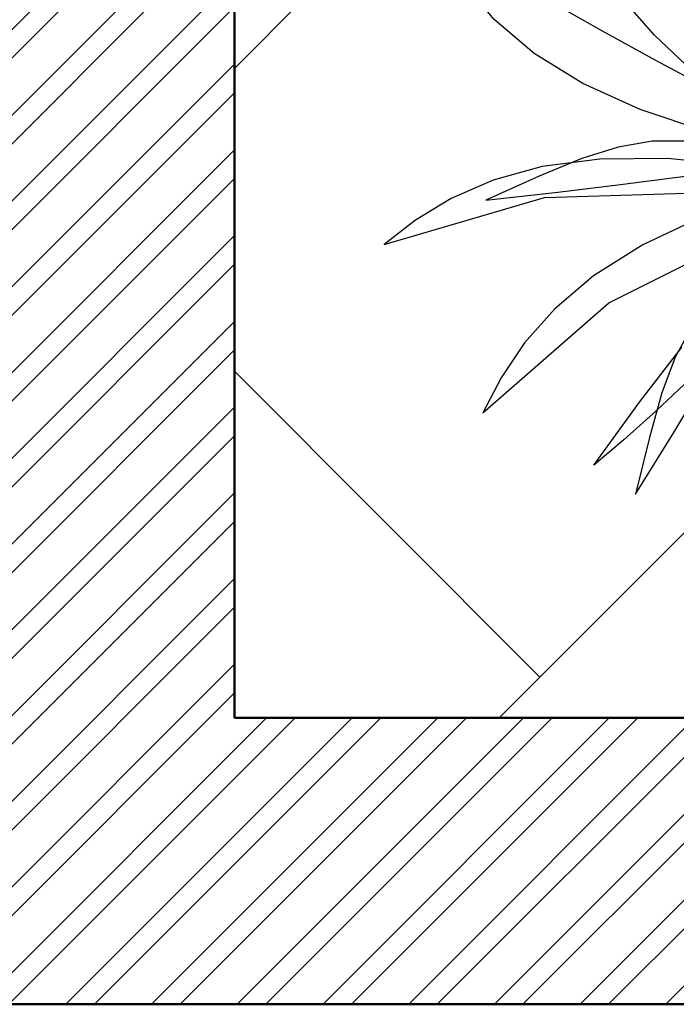
# Model space of a CAD drawing. Units: inches. Extents: x 3590 to 5167, y 65 to 1917.
# Tile 29 of 100: x 4927 to 4947, y 1326 to 1357. Entities that reach past the tile are written whole.
import ezdxf

# ---------------------------------------------------------------- set-up
doc = ezdxf.new("R2010")
doc.units = ezdxf.units.IN
for name, color, linetype, lineweight in [('A-FLOR-PATT', 8, 'Continuous', 13), ('A-WALL', 7, 'Continuous', 50), ('A-WALL-PATT', 251, 'Continuous', 13), ('L-PLNT', 94, 'Continuous', 18)]:
    doc.layers.add(name, color=color, linetype=linetype, lineweight=lineweight)
doc.layers.add('DIENHOA', color=3, linetype='Continuous')

# ---------------------------------------------------------------- blocks, each defined once
blk = doc.blocks.new('Cay03_mb')
at = {"layer": 'DIENHOA'}
for p, q in [((-254.7, 27.4), (-298.6, 20.1)), ((-208, 27.8), (-254.7, 27.4)), ((-298.6, 20.1), (-345, 5.4)), ((-345, 5.4), (-399.6, -17.1)), ((-225.8, -18.9), (-165.8, -11.3)), ((-399.6, -17.1), (-468, -47.9)), ((-295.3, -27.9), (-225.8, -18.9)), ((-468, -47.9), (-375.6, -37.8)), ((-375.6, -37.8), (-295.3, -27.9)), ((-271, -306.6), (-216.3, -235.6)), ((-206.3, -276.5), (-249.6, -317.8)), ((-329.5, -387.1), (-271, -306.6)), ((-249.6, -317.8), (-291, -354.7)), ((-291, -354.7), (-329.5, -387.1))]:
    blk.add_line(p, q, dxfattribs=at)
for points in [[(-16.4, -26.7), (-108.3, 38.6), (-186.9, 101.7), (-252.4, 163.5), (-305.1, 224.4), (-345.4, 285.2), (-373.7, 346.6), (-390.4, 409.2), (-395.6, 473.7)], [(-530.5, 289.7), (-458.3, 248.1), (-387.9, 207.8), (-318.9, 168.7), (-250.8, 131.1), (-182.9, 94.8), (-114.9, 59.9), (-46.2, 26.5), (23.7, -5.4)], [(23.7, -5.4), (-87.2, 15.2), (-185, 39.6), (-270.3, 68.2), (-343.7, 101.4), (-405.9, 139.7), (-457.3, 183.5), (-498.7, 233.4), (-530.5, 289.7)], [(-16.4, -26.7), (-134, -4.7), (-235.3, 5.3), (-322, 4.7), (-395.9, -5), (-458.7, -22.3), (-512.3, -45.7), (-558.2, -73.6), (-598.4, -104.7)], [(-471.9, -320.3), (-310.5, -179.3), (-97.7, -73.3), (23.7, -5.4)], [(23.7, -5.4), (-92.3, -34.8), (-188.4, -68.2), (-266.9, -105.1), (-329.9, -144.9), (-379.7, -187), (-418.5, -230.7), (-448.5, -275.3), (-471.9, -320.3)], [(-598.4, -104.7), (-392.7, -44.4), (-155, -37.4), (-16.4, -26.7)], [(-276.2, -424.4), (-227.3, -345.4), (-185.7, -276.1), (-150, -215.7), (-119.1, -163.8), (-91.5, -119.5), (-66, -82.3), (-41.4, -51.6), (-16.4, -26.7)], [(-16.4, -26.7), (-84.9, -86), (-137, -133.1), (-175.8, -173), (-204.3, -210), (-225.5, -249.1), (-242.5, -294.7), (-258.4, -351.6), (-276.2, -424.4)]]:
    blk.add_lwpolyline(points, dxfattribs=at)

msp = doc.modelspace()

# ---------------------------------------------------------------- hatches: boundary and pattern name
at = {"layer": 'A-FLOR-PATT', "transparency": 33554687}
h = msp.add_hatch(dxfattribs=at)
h.set_pattern_fill('AR-HBONE', color=256, scale=0.2)
h.set_pattern_definition([(45, (-588.972, 0), (0, 28.73682), [60.96, -20.32]), (135, (-574.604, 14.368), (3e-15, 28.73682), [60.96, -20.32])])
h.paths.add_polyline_path([(5071.274, 1796.999), (4933.274, 1796.999), (4933.274, 1753.999), (4962.774, 1753.999, -0.414214), (4928.774, 1719.999), (4933.274, 1718.999), (4933.274, 1334.999), (5071.274, 1334.999)])
h.paths.add_polyline_path([(4951.78, 1521.077), (4951.715, 1521.04), (4951.563, 1520.895)], flags=16)
h.paths.add_polyline_path([(4952.267, 1521.376), (4952.198, 1521.371), (4952.198, 1521.356)], flags=0)
h.paths.add_polyline_path([(4967.051, 1529.728), (4965.231, 1528.694), (4963.411, 1527.714), (4961.756, 1526.851), (4963.589, 1527.449), (4964.036, 1527.478), (4962.975, 1527.249), (4961.76, 1526.852), (4959.792, 1525.834), (4958.005, 1524.895), (4956.24, 1523.93), (4954.504, 1522.919), (4954.129, 1522.682), (4953.361, 1521.997), (4953.366, 1521.998), (4953.605, 1522.064), (4955.106, 1522.761), (4956.921, 1523.434), (4958.678, 1523.915), (4960.358, 1524.2), (4961.945, 1524.286), (4964.171, 1524.108), (4965.958, 1523.309), (4963.863, 1522.976), (4965.187, 1522.499), (4963.366, 1522.497), (4961.545, 1522.487), (4959.764, 1522.461), (4958.304, 1522.419), (4957.974, 1522.388), (4956.307, 1522.232), (4954.718, 1522.071), (4953.251, 1521.899), (4953.525, 1521.623), (4954.331, 1521.379), (4956.243, 1521.23), (4958.039, 1520.93), (4959.684, 1520.483), (4961.16, 1519.896), (4963.107, 1518.8), (4964.393, 1517.325), (4962.973, 1517.726), (4964.558, 1516.661), (4965.407, 1515.708), (4963.507, 1516.322), (4961.68, 1517.005), (4959.935, 1517.745), (4958.282, 1518.528), (4956.732, 1519.343), (4955.295, 1520.175), (4954.672, 1520.572), (4954.513, 1520.627), (4955.658, 1519.318), (4956.703, 1517.982), (4957.644, 1516.647), (4958.485, 1515.334), (4959.55, 1513.524), (4960.438, 1511.769), (4958.841, 1513.62), (4957.452, 1515.325), (4955.819, 1517.459), (4956.665, 1515.448), (4957.111, 1513.923), (4957.447, 1511.714), (4957.076, 1509.793), (4956.538, 1511.11), (4955.992, 1512.569), (4955.444, 1514.125), (4954.898, 1515.735), (4954.357, 1517.356), (4953.824, 1518.943), (4953.305, 1520.452), (4953.065, 1521.116), (4952.971, 1521.146), (4952.949, 1521.086), (4952.73, 1520.199), (4953.37, 1518.024), (4953.757, 1516.373), (4954.051, 1514.765), (4954.264, 1513.221), (4954.471, 1511.131), (4954.497, 1510.402), (4954.409, 1511.76), (4954.264, 1513.221), (4954.051, 1514.765), (4953.757, 1516.373), (4953.37, 1518.024), (4952.877, 1519.698), (4952.716, 1520.141), (4952.533, 1519.059), (4952.374, 1517.789), (4952.219, 1516.312), (4952.046, 1514.6), (4951.833, 1512.626), (4951.557, 1510.363), (4951.203, 1512.168), (4950.852, 1514.339), (4950.985, 1516.376), (4951.66, 1518.286), (4952.593, 1520.481), (4952.357, 1521.13), (4951.855, 1520.328), (4950.839, 1518.908), (4949.777, 1517.587), (4948.916, 1516.617), (4948.111, 1515.256), (4947.089, 1513.554), (4945.889, 1511.615), (4946.326, 1513.402), (4946.562, 1514.249), (4945.528, 1513.327), (4944.581, 1512.531), (4946.018, 1514.508), (4947.204, 1516.048), (4947.893, 1517.313), (4949.307, 1518.764), (4950.414, 1519.767), (4950.451, 1519.806), (4952.267, 1521.376), (4951.645, 1521.493), (4950.404, 1521.18), (4948.044, 1520.359), (4946.119, 1519.452), (4944.572, 1518.475), (4943.35, 1517.443), (4941.997, 1515.92), (4941.661, 1515.275), (4942.813, 1516.99), (4944.572, 1518.475), (4946.119, 1519.452), (4948.044, 1520.359), (4950.404, 1521.18), (4951.645, 1521.493), (4949.647, 1521.868), (4948.6, 1521.756), (4947.126, 1521.57), (4945.42, 1521.348), (4943.45, 1521.105), (4941.183, 1520.856), (4942.86, 1521.613), (4943.873, 1522.03), (4942.952, 1521.909), (4941.41, 1521.485), (4939.543, 1520.67), (4938.968, 1520.226), (4940.733, 1521.299), (4942.952, 1521.909), (4943.702, 1522.008), (4945.894, 1522.7), (4947.565, 1522.714), (4948.921, 1522.566), (4951.131, 1522.183), (4950.971, 1522.297), (4948.129, 1523.006), (4946.035, 1523.707), (4944.232, 1524.521), (4942.707, 1525.461), (4941.444, 1526.537), (4940.43, 1527.761), (4939.649, 1529.143), (4941.421, 1528.122), (4943.147, 1527.132), (4944.841, 1526.175), (4946.514, 1525.25), (4948.179, 1524.359), (4948.365, 1524.263), (4946.475, 1526.045), (4945.181, 1527.54), (4944.19, 1529.033), (4943.496, 1530.54), (4943.278, 1531.36), (4942.498, 1531.919), (4943.114, 1531.762), (4942.959, 1533.659), (4944.14, 1531.989), (4944.612, 1531.323), (4946.202, 1530.463), (4947.486, 1529.509), (4948.79, 1528.226), (4950.368, 1526.237), (4949.485, 1528.155), (4948.851, 1530.123), (4948.491, 1532.041), (4948.381, 1533.918), (4948.501, 1535.76), (4948.827, 1537.573), (4949.418, 1535.565), (4949.957, 1533.569), (4950.464, 1531.586), (4950.961, 1529.617), (4951.391, 1527.954), (4951.724, 1530.687), (4952.201, 1532.58), (4952.889, 1534.33), (4953.77, 1535.951), (4954.827, 1537.46), (4954.521, 1535.39), (4954.273, 1533.937), (4955.58, 1535.663), (4956.748, 1536.739), (4956.159, 1534.78), (4955.589, 1532.873), (4955.043, 1531.006), (4954.525, 1529.166), (4954.038, 1527.341), (4953.638, 1525.733), (4953.611, 1525.586), (4953.398, 1524.166), (4953.382, 1524.009), (4954.07, 1525.476), (4954.912, 1527.022), (4956.136, 1528.894), (4957.847, 1530.577), (4959.376, 1531.54), (4958.256, 1530.104), (4957.143, 1528.663), (4956.066, 1527.243), (4955.056, 1525.871), (4954.141, 1524.571), (4953.352, 1523.372), (4953.311, 1523.303), (4953.273, 1522.925), (4953.261, 1522.382), (4954.103, 1523.373), (4954.63, 1524.284), (4955.961, 1526.358), (4957.23, 1528.13), (4958.421, 1529.609), (4960.037, 1531.368), (4961.374, 1532.375), (4962.101, 1532.77), (4961.07, 1531.061), (4959.987, 1529.438), (4958.869, 1527.908), (4958.15, 1527.007), (4959.803, 1528.003), (4961.589, 1528.793), (4963.391, 1529.328), (4965.211, 1529.632)], flags=16)
h.paths.add_polyline_path([(4962.944, 1523.182), (4961.107, 1523.422), (4960.392, 1523.362), (4962.35, 1523.331)], flags=0)
h.paths.add_polyline_path([(5049.541, 1584.551), (5049.476, 1584.515), (5049.325, 1584.37)], flags=16)
h.paths.add_polyline_path([(5050.028, 1584.851), (5049.959, 1584.845), (5049.959, 1584.83)], flags=0)
h.paths.add_polyline_path([(5042.333, 1581.949), (5043.88, 1582.926), (5045.806, 1583.833), (5048.165, 1584.654), (5049.406, 1584.967), (5047.408, 1585.342), (5046.361, 1585.231), (5044.888, 1585.044), (5043.181, 1584.822), (5041.211, 1584.579), (5038.944, 1584.33), (5040.622, 1585.087), (5041.634, 1585.504), (5040.713, 1585.383), (5039.171, 1584.959), (5037.304, 1584.144), (5036.729, 1583.7), (5038.494, 1584.773), (5040.713, 1585.383), (5041.463, 1585.482), (5043.655, 1586.174), (5045.326, 1586.188), (5046.682, 1586.04), (5048.893, 1585.657), (5048.732, 1585.771), (5045.891, 1586.48), (5043.796, 1587.181), (5041.994, 1587.996), (5040.468, 1588.935), (5039.205, 1590.011), (5038.191, 1591.235), (5037.41, 1592.617), (5039.182, 1591.596), (5040.909, 1590.607), (5042.602, 1589.649), (5044.275, 1588.724), (5045.94, 1587.833), (5046.126, 1587.738), (5044.237, 1589.519), (5042.942, 1591.015), (5041.952, 1592.508), (5041.257, 1594.014), (5041.039, 1594.834), (5040.26, 1595.393), (5040.875, 1595.237), (5040.721, 1597.133), (5041.901, 1595.463), (5042.373, 1594.798), (5043.963, 1593.938), (5045.247, 1592.983), (5046.552, 1591.701), (5048.129, 1589.712), (5047.247, 1591.63), (5046.613, 1593.597), (5046.252, 1595.515), (5046.142, 1597.392), (5046.262, 1599.234), (5046.588, 1601.047), (5047.179, 1599.039), (5047.718, 1597.043), (5048.225, 1595.06), (5048.722, 1593.091), (5049.152, 1591.429), (5049.485, 1594.161), (5049.962, 1596.054), (5050.65, 1597.804), (5051.532, 1599.425), (5052.589, 1600.934), (5052.283, 1598.864), (5052.034, 1597.411), (5053.341, 1599.137), (5054.509, 1600.213), (5053.92, 1598.254), (5053.35, 1596.348), (5052.805, 1594.48), (5052.286, 1592.64), (5051.799, 1590.815), (5051.4, 1589.207), (5051.373, 1589.06), (5051.159, 1587.64), (5051.143, 1587.483), (5051.831, 1588.95), (5052.673, 1590.496), (5053.898, 1592.368), (5055.608, 1594.051), (5057.137, 1595.014), (5056.017, 1593.578), (5054.904, 1592.137), (5053.828, 1590.717), (5052.817, 1589.345), (5051.902, 1588.046), (5051.113, 1586.846), (5051.072, 1586.777), (5051.034, 1586.399), (5051.022, 1585.856), (5051.864, 1586.847), (5052.391, 1587.758), (5053.723, 1589.832), (5054.991, 1591.604), (5056.182, 1593.083), (5057.798, 1594.842), (5059.135, 1595.849), (5059.863, 1596.244), (5058.831, 1594.535), (5057.749, 1592.912), (5056.63, 1591.382), (5055.912, 1590.482), (5057.564, 1591.477), (5059.35, 1592.267), (5061.152, 1592.802), (5062.972, 1593.106), (5064.812, 1593.203), (5062.992, 1592.169), (5061.172, 1591.188), (5059.518, 1590.325), (5061.35, 1590.924), (5061.797, 1590.952), (5060.737, 1590.723), (5059.521, 1590.326), (5057.553, 1589.308), (5055.766, 1588.369), (5054.002, 1587.404), (5052.265, 1586.393), (5051.891, 1586.156), (5051.122, 1585.471), (5051.127, 1585.472), (5051.366, 1585.538), (5052.867, 1586.235), (5054.682, 1586.908), (5056.439, 1587.389), (5058.12, 1587.675), (5059.706, 1587.76), (5061.933, 1587.583), (5063.719, 1586.783), (5061.624, 1586.45), (5062.949, 1585.973), (5061.127, 1585.971), (5059.307, 1585.961), (5057.525, 1585.935), (5056.065, 1585.893), (5055.735, 1585.862), (5054.068, 1585.707), (5052.479, 1585.546), (5051.012, 1585.373), (5051.286, 1585.097), (5052.092, 1584.853), (5054.004, 1584.704), (5055.8, 1584.404), (5057.446, 1583.958), (5058.921, 1583.37), (5060.868, 1582.274), (5062.154, 1580.799), (5060.734, 1581.2), (5062.32, 1580.135), (5063.168, 1579.182), (5061.269, 1579.796), (5059.441, 1580.479), (5057.696, 1581.219), (5056.043, 1582.003), (5054.493, 1582.817), (5053.057, 1583.649), (5052.433, 1584.047), (5052.274, 1584.101), (5053.42, 1582.793), (5054.464, 1581.457), (5055.405, 1580.121), (5056.247, 1578.809), (5057.311, 1576.998), (5058.199, 1575.244), (5056.602, 1577.094), (5055.213, 1578.799), (5053.58, 1580.933), (5054.427, 1578.922), (5054.872, 1577.397), (5055.208, 1575.189), (5054.838, 1573.267), (5054.299, 1574.584), (5053.754, 1576.043), (5053.206, 1577.599), (5052.659, 1579.209), (5052.118, 1580.83), (5051.585, 1582.417), (5051.066, 1583.927), (5050.826, 1584.59), (5050.733, 1584.62), (5050.711, 1584.561), (5050.491, 1583.673), (5051.131, 1581.498), (5051.518, 1579.847), (5051.813, 1578.24), (5052.026, 1576.695), (5052.233, 1574.605), (5052.258, 1573.876), (5052.17, 1575.234), (5052.026, 1576.695), (5051.813, 1578.24), (5051.518, 1579.847), (5051.131, 1581.498), (5050.638, 1583.172), (5050.477, 1583.615), (5050.294, 1582.533), (5050.136, 1581.263), (5049.981, 1579.786), (5049.807, 1578.074), (5049.594, 1576.1), (5049.318, 1573.837), (5048.965, 1575.642), (5048.613, 1577.813), (5048.747, 1579.85), (5049.421, 1581.76), (5050.354, 1583.955), (5050.118, 1584.604), (5049.616, 1583.802), (5048.6, 1582.382), (5047.538, 1581.061), (5046.677, 1580.091), (5045.872, 1578.73), (5044.85, 1577.028), (5043.651, 1575.089), (5044.087, 1576.877), (5044.324, 1577.723), (5043.289, 1576.801), (5042.342, 1576.005), (5043.779, 1577.982), (5044.966, 1579.522), (5045.655, 1580.787), (5047.068, 1582.239), (5048.175, 1583.241), (5048.213, 1583.28), (5050.028, 1584.851), (5049.406, 1584.967), (5048.165, 1584.654), (5045.806, 1583.833), (5043.88, 1582.926), (5042.333, 1581.949), (5041.111, 1580.917), (5039.758, 1579.394), (5039.423, 1578.749), (5040.575, 1580.464)], flags=16)
h.paths.add_polyline_path([(4954.799, 1533.12), (4954.262, 1532.079), (4953.831, 1530.935), (4953.505, 1529.636), (4953.283, 1528.133), (4953.167, 1526.376), (4953.156, 1524.315), (4953.277, 1521.236), (4952.802, 1521.842), (4951.557, 1521.998), (4950.976, 1521.961), (4952.661, 1521.941), (4952.802, 1521.842), (4953.152, 1523.593), (4953.167, 1526.376), (4953.283, 1528.133), (4953.609, 1530.346), (4954.456, 1532.592)], flags=0)
h.paths.add_polyline_path([(5050.563, 1585.316), (5049.318, 1585.472), (5048.737, 1585.435), (5050.422, 1585.415), (5050.563, 1585.316), (5050.914, 1587.067), (5050.928, 1589.851), (5051.045, 1591.607), (5051.371, 1593.82), (5052.217, 1596.066), (5052.56, 1596.594), (5052.024, 1595.554), (5051.592, 1594.409), (5051.266, 1593.11), (5051.045, 1591.607), (5050.928, 1589.851), (5050.918, 1587.789), (5051.038, 1584.71)], flags=0)
h.paths.add_polyline_path([(5058.153, 1586.836), (5060.111, 1586.805), (5060.705, 1586.656), (5058.868, 1586.896)], flags=0)
h.paths.add_polyline_path([(5049.541, 1430.936), (5049.476, 1430.9), (5049.325, 1430.755)], flags=16)
h.paths.add_polyline_path([(5050.028, 1431.236), (5049.959, 1431.231), (5049.959, 1431.215)], flags=0)
h.paths.add_polyline_path([(5046.588, 1447.432), (5047.179, 1445.425), (5047.718, 1443.429), (5048.225, 1441.446), (5048.722, 1439.476), (5049.152, 1437.814), (5049.485, 1440.546), (5049.962, 1442.439), (5050.65, 1444.189), (5051.532, 1445.811), (5052.589, 1447.319), (5052.283, 1445.249), (5052.034, 1443.796), (5053.341, 1445.522), (5054.509, 1446.598), (5053.92, 1444.64), (5053.35, 1442.733), (5052.805, 1440.865), (5052.286, 1439.025), (5051.799, 1437.201), (5051.4, 1435.592), (5051.373, 1435.445), (5051.159, 1434.025), (5051.143, 1433.868), (5051.831, 1435.335), (5052.673, 1436.881), (5053.898, 1438.753), (5055.608, 1440.436), (5057.137, 1441.4), (5056.017, 1439.963), (5054.904, 1438.522), (5053.828, 1437.102), (5052.817, 1435.73), (5051.902, 1434.431), (5051.113, 1433.231), (5051.072, 1433.162), (5051.034, 1432.784), (5051.022, 1432.242), (5051.864, 1433.232), (5052.391, 1434.143), (5053.723, 1436.217), (5054.991, 1437.989), (5056.182, 1439.468), (5057.798, 1441.227), (5059.135, 1442.235), (5059.863, 1442.629), (5058.831, 1440.921), (5057.749, 1439.298), (5056.63, 1437.767), (5055.912, 1436.867), (5057.564, 1437.863), (5059.35, 1438.652), (5061.152, 1439.187), (5062.972, 1439.491), (5064.812, 1439.588), (5062.992, 1438.554), (5061.172, 1437.573), (5059.518, 1436.71), (5061.35, 1437.309), (5061.797, 1437.337), (5060.737, 1437.108), (5059.521, 1436.711), (5057.553, 1435.693), (5055.766, 1434.754), (5054.002, 1433.789), (5052.265, 1432.778), (5051.891, 1432.541), (5051.122, 1431.856), (5051.127, 1431.857), (5051.366, 1431.923), (5052.867, 1432.62), (5054.682, 1433.293), (5056.439, 1433.775), (5058.12, 1434.06), (5059.706, 1434.145), (5061.933, 1433.968), (5063.719, 1433.168), (5061.624, 1432.835), (5062.949, 1432.358), (5061.127, 1432.357), (5059.307, 1432.346), (5057.525, 1432.32), (5056.065, 1432.278), (5055.735, 1432.248), (5054.068, 1432.092), (5052.479, 1431.931), (5051.012, 1431.759), (5051.286, 1431.482), (5052.092, 1431.238), (5054.004, 1431.089), (5055.8, 1430.789), (5057.446, 1430.343), (5058.921, 1429.755), (5060.868, 1428.66), (5062.154, 1427.185), (5060.734, 1427.585), (5062.32, 1426.52), (5063.168, 1425.567), (5061.269, 1426.181), (5059.441, 1426.865), (5057.696, 1427.604), (5056.043, 1428.388), (5054.493, 1429.202), (5053.057, 1430.034), (5052.433, 1430.432), (5052.274, 1430.487), (5053.42, 1429.178), (5054.464, 1427.842), (5055.405, 1426.506), (5056.247, 1425.194), (5057.311, 1423.383), (5058.199, 1421.629), (5056.602, 1423.479), (5055.213, 1425.184), (5053.58, 1427.318), (5054.427, 1425.307), (5054.872, 1423.782), (5055.208, 1421.574), (5054.838, 1419.652), (5054.299, 1420.97), (5053.754, 1422.428), (5053.206, 1423.984), (5052.659, 1425.595), (5052.118, 1427.215), (5051.585, 1428.802), (5051.066, 1430.312), (5050.826, 1430.975), (5050.733, 1431.005), (5050.711, 1430.946), (5050.491, 1430.058), (5051.131, 1427.883), (5051.518, 1426.232), (5051.813, 1424.625), (5052.026, 1423.081), (5052.233, 1420.991), (5052.258, 1420.261), (5052.17, 1421.619), (5052.026, 1423.081), (5051.813, 1424.625), (5051.518, 1426.232), (5051.131, 1427.883), (5050.638, 1429.558), (5050.477, 1430.001), (5050.294, 1428.918), (5050.136, 1427.648), (5049.981, 1426.171), (5049.807, 1424.459), (5049.594, 1422.485), (5049.318, 1420.222), (5048.965, 1422.028), (5048.613, 1424.199), (5048.747, 1426.235), (5049.421, 1428.146), (5050.354, 1430.34), (5050.118, 1430.989), (5049.616, 1430.187), (5048.6, 1428.768), (5047.538, 1427.446), (5046.677, 1426.477), (5045.872, 1425.116), (5044.85, 1423.413), (5043.651, 1421.474), (5044.087, 1423.262), (5044.324, 1424.109), (5043.289, 1423.186), (5042.342, 1422.391), (5043.779, 1424.368), (5044.966, 1425.907), (5045.655, 1427.173), (5047.068, 1428.624), (5048.175, 1429.627), (5048.213, 1429.666), (5050.028, 1431.236), (5049.406, 1431.353), (5048.165, 1431.039), (5045.806, 1430.218), (5043.88, 1429.311), (5042.333, 1428.334), (5041.111, 1427.302), (5039.758, 1425.779), (5039.423, 1425.134), (5040.575, 1426.849), (5042.333, 1428.334), (5043.88, 1429.311), (5045.806, 1430.218), (5048.165, 1431.039), (5049.406, 1431.353), (5047.408, 1431.727), (5046.361, 1431.616), (5044.888, 1431.429), (5043.181, 1431.207), (5041.211, 1430.964), (5038.944, 1430.715), (5040.622, 1431.472), (5041.634, 1431.89), (5040.713, 1431.769), (5039.171, 1431.345), (5037.304, 1430.53), (5036.729, 1430.085), (5038.494, 1431.158), (5040.713, 1431.769), (5041.463, 1431.867), (5043.655, 1432.559), (5045.326, 1432.573), (5046.682, 1432.425), (5048.893, 1432.042), (5048.732, 1432.156), (5045.891, 1432.865), (5043.796, 1433.566), (5041.994, 1434.381), (5040.468, 1435.321), (5039.205, 1436.396), (5038.191, 1437.62), (5037.41, 1439.002), (5039.182, 1437.982), (5040.909, 1436.992), (5042.602, 1436.034), (5044.275, 1435.109), (5045.94, 1434.218), (5046.126, 1434.123), (5044.237, 1435.904), (5042.942, 1437.4), (5041.952, 1438.893), (5041.257, 1440.399), (5041.039, 1441.219), (5040.26, 1441.778), (5040.875, 1441.622), (5040.721, 1443.518), (5041.901, 1441.848), (5042.373, 1441.183), (5043.963, 1440.323), (5045.247, 1439.369), (5046.552, 1438.086), (5048.129, 1436.097), (5047.247, 1438.015), (5046.613, 1439.982), (5046.252, 1441.901), (5046.142, 1443.778), (5046.262, 1445.619)], flags=16)
h.paths.add_polyline_path([(5052.382, 1444.255), (5051.623, 1442.78), (5052.024, 1441.939), (5052.56, 1442.98)], flags=0)
h.paths.add_polyline_path([(5050.563, 1431.701), (5049.318, 1431.857), (5048.737, 1431.821), (5050.422, 1431.8)], flags=0)
h.paths.add_polyline_path([(5058.153, 1433.221), (5060.111, 1433.19), (5060.705, 1433.041), (5058.868, 1433.281)], flags=0)
h.paths.add_polyline_path([(5049.541, 1352.285), (5049.476, 1352.249), (5049.325, 1352.104)], flags=16)
h.paths.add_polyline_path([(5050.028, 1352.585), (5049.959, 1352.58), (5049.959, 1352.564)], flags=0)
h.paths.add_polyline_path([(5046.588, 1368.781), (5047.179, 1366.774), (5047.718, 1364.778), (5048.225, 1362.795), (5048.722, 1360.825), (5049.152, 1359.163), (5049.485, 1361.896), (5049.962, 1363.789), (5050.65, 1365.538), (5051.532, 1367.16), (5052.589, 1368.669), (5052.283, 1366.598), (5052.034, 1365.145), (5053.341, 1366.871), (5054.509, 1367.947), (5053.92, 1365.989), (5053.35, 1364.082), (5052.805, 1362.214), (5052.286, 1360.374), (5051.799, 1358.55), (5051.4, 1356.942), (5051.373, 1356.794), (5051.159, 1355.374), (5051.143, 1355.218), (5051.831, 1356.684), (5052.673, 1358.23), (5053.898, 1360.102), (5055.608, 1361.786), (5057.137, 1362.749), (5056.017, 1361.313), (5054.904, 1359.872), (5053.828, 1358.452), (5052.817, 1357.079), (5051.902, 1355.78), (5051.113, 1354.581), (5051.072, 1354.512), (5051.034, 1354.133), (5051.022, 1353.591), (5051.864, 1354.581), (5052.391, 1355.492), (5053.723, 1357.566), (5054.991, 1359.338), (5056.182, 1360.817), (5057.798, 1362.577), (5059.135, 1363.584), (5059.863, 1363.979), (5058.831, 1362.27), (5057.749, 1360.647), (5056.63, 1359.117), (5055.912, 1358.216), (5057.564, 1359.212), (5059.35, 1360.001), (5061.152, 1360.536), (5062.972, 1360.841), (5064.812, 1360.937), (5062.992, 1359.903), (5061.172, 1358.923), (5059.518, 1358.059), (5061.35, 1358.658), (5061.797, 1358.687), (5060.737, 1358.458), (5059.521, 1358.061), (5057.553, 1357.043), (5055.766, 1356.103), (5054.002, 1355.138), (5052.265, 1354.127), (5051.891, 1353.89), (5051.122, 1353.206), (5051.127, 1353.206), (5051.366, 1353.272), (5052.867, 1353.969), (5054.682, 1354.643), (5056.439, 1355.124), (5058.12, 1355.409), (5059.706, 1355.495), (5061.933, 1355.317), (5063.719, 1354.518), (5061.624, 1354.184), (5062.949, 1353.708), (5061.127, 1353.706), (5059.307, 1353.695), (5057.525, 1353.669), (5056.065, 1353.627), (5055.735, 1353.597), (5054.068, 1353.441), (5052.479, 1353.28), (5051.012, 1353.108), (5051.286, 1352.831), (5052.092, 1352.587), (5054.004, 1352.439), (5055.8, 1352.138), (5057.446, 1351.692), (5058.921, 1351.104), (5060.868, 1350.009), (5062.154, 1348.534), (5060.734, 1348.935), (5062.32, 1347.869), (5063.168, 1346.916), (5061.269, 1347.53), (5059.441, 1348.214), (5057.696, 1348.954), (5056.043, 1349.737), (5054.493, 1350.551), (5053.057, 1351.383), (5052.433, 1351.781), (5052.274, 1351.836), (5053.42, 1350.527), (5054.464, 1349.191), (5055.405, 1347.855), (5056.247, 1346.543), (5057.311, 1344.733), (5058.199, 1342.978), (5056.602, 1344.828), (5055.213, 1346.534), (5053.58, 1348.667), (5054.427, 1346.656), (5054.872, 1345.132), (5055.208, 1342.923), (5054.838, 1341.002), (5054.299, 1342.319), (5053.754, 1343.778), (5053.206, 1345.334), (5052.659, 1346.944), (5052.118, 1348.564), (5051.585, 1350.151), (5051.066, 1351.661), (5050.826, 1352.324), (5050.733, 1352.355), (5050.711, 1352.295), (5050.491, 1351.408), (5051.131, 1349.232), (5051.518, 1347.581), (5051.813, 1345.974), (5052.026, 1344.43), (5052.233, 1342.34), (5052.258, 1341.61), (5052.17, 1342.969), (5052.026, 1344.43), (5051.813, 1345.974), (5051.518, 1347.581), (5051.131, 1349.232), (5050.638, 1350.907), (5050.477, 1351.35), (5050.294, 1350.267), (5050.136, 1348.997), (5049.981, 1347.52), (5049.807, 1345.809), (5049.594, 1343.835), (5049.318, 1341.571), (5048.965, 1343.377), (5048.613, 1345.548), (5048.747, 1347.585), (5049.421, 1349.495), (5050.354, 1351.689), (5050.118, 1352.339), (5049.616, 1351.536), (5048.6, 1350.117), (5047.538, 1348.795), (5046.677, 1347.826), (5045.872, 1346.465), (5044.85, 1344.763), (5043.651, 1342.824), (5044.087, 1344.611), (5044.324, 1345.458), (5043.289, 1344.535), (5042.342, 1343.74), (5043.779, 1345.717), (5044.966, 1347.256), (5045.655, 1348.522), (5047.068, 1349.973), (5048.175, 1350.976), (5048.213, 1351.015), (5050.028, 1352.585), (5049.406, 1352.702), (5048.165, 1352.388), (5045.806, 1351.567), (5043.88, 1350.661), (5042.333, 1349.683), (5041.111, 1348.651), (5039.758, 1347.128), (5039.423, 1346.483), (5040.575, 1348.198), (5042.333, 1349.683), (5043.88, 1350.661), (5045.806, 1351.567), (5048.165, 1352.388), (5049.406, 1352.702), (5047.408, 1353.076), (5046.361, 1352.965), (5044.888, 1352.779), (5043.181, 1352.556), (5041.211, 1352.313), (5038.944, 1352.065), (5040.622, 1352.821), (5041.634, 1353.239), (5040.713, 1353.118), (5039.171, 1352.694), (5037.304, 1351.879), (5036.729, 1351.434), (5038.494, 1352.508), (5040.713, 1353.118), (5041.463, 1353.216), (5043.655, 1353.909), (5045.326, 1353.923), (5046.682, 1353.774), (5048.893, 1353.391), (5048.732, 1353.506), (5045.891, 1354.214), (5043.796, 1354.915), (5041.994, 1355.73), (5040.468, 1356.67), (5039.205, 1357.746), (5038.191, 1358.969), (5037.41, 1360.352), (5039.182, 1359.331), (5040.909, 1358.341), (5042.602, 1357.383), (5044.275, 1356.458), (5045.94, 1355.567), (5046.126, 1355.472), (5044.237, 1357.253), (5042.942, 1358.749), (5041.952, 1360.242), (5041.257, 1361.748), (5041.039, 1362.568), (5040.26, 1363.128), (5040.875, 1362.971), (5040.721, 1364.867), (5041.901, 1363.197), (5042.373, 1362.532), (5043.963, 1361.672), (5045.247, 1360.718), (5046.552, 1359.435), (5048.129, 1357.446), (5047.247, 1359.364), (5046.613, 1361.331), (5046.252, 1363.25), (5046.142, 1365.127), (5046.262, 1366.969)], flags=16)
h.paths.add_polyline_path([(5052.382, 1365.604), (5051.623, 1364.129), (5052.024, 1363.288), (5052.56, 1364.329)], flags=0)
h.paths.add_polyline_path([(4951.78, 1698.041), (4951.715, 1698.005), (4951.563, 1697.859)], flags=16)
h.paths.add_polyline_path([(4952.267, 1698.341), (4952.198, 1698.335), (4952.198, 1698.32)], flags=0)
h.paths.add_polyline_path([(4957.076, 1686.757), (4956.538, 1688.074), (4955.992, 1689.533), (4955.444, 1691.089), (4954.898, 1692.699), (4954.357, 1694.32), (4953.824, 1695.907), (4953.305, 1697.417), (4953.065, 1698.08), (4952.971, 1698.11), (4952.949, 1698.051), (4952.73, 1697.163), (4953.37, 1694.988), (4953.757, 1693.337), (4954.051, 1691.729), (4954.264, 1690.185), (4954.471, 1688.095), (4954.497, 1687.366), (4954.409, 1688.724), (4954.264, 1690.185), (4954.051, 1691.729), (4953.757, 1693.337), (4953.37, 1694.988), (4952.877, 1696.662), (4952.716, 1697.105), (4952.533, 1696.023), (4952.374, 1694.753), (4952.219, 1693.276), (4952.046, 1691.564), (4951.833, 1689.59), (4951.557, 1687.327), (4951.203, 1689.132), (4950.852, 1691.303), (4950.985, 1693.34), (4951.66, 1695.25), (4952.593, 1697.445), (4952.357, 1698.094), (4951.855, 1697.292), (4950.839, 1695.872), (4949.777, 1694.551), (4948.916, 1693.581), (4948.111, 1692.22), (4947.089, 1690.518), (4945.889, 1688.579), (4946.326, 1690.366), (4946.562, 1691.213), (4945.528, 1690.291), (4944.581, 1689.495), (4946.018, 1691.472), (4947.204, 1693.012), (4947.893, 1694.277), (4949.307, 1695.729), (4950.414, 1696.731), (4950.451, 1696.77), (4952.267, 1698.341), (4951.645, 1698.457), (4950.404, 1698.144), (4948.044, 1697.323), (4946.119, 1696.416), (4944.572, 1695.439), (4943.35, 1694.407), (4941.997, 1692.884), (4941.661, 1692.239), (4942.813, 1693.954), (4944.572, 1695.439), (4946.119, 1696.416), (4948.044, 1697.323), (4950.404, 1698.144), (4951.645, 1698.457), (4949.647, 1698.832), (4948.6, 1698.72), (4947.126, 1698.534), (4945.42, 1698.312), (4943.45, 1698.069), (4941.183, 1697.82), (4942.86, 1698.577), (4943.873, 1698.994), (4942.952, 1698.873), (4941.41, 1698.449), (4939.543, 1697.634), (4938.968, 1697.19), (4940.733, 1698.263), (4942.952, 1698.873), (4943.702, 1698.972), (4945.894, 1699.664), (4947.565, 1699.678), (4948.921, 1699.53), (4951.131, 1699.147), (4950.971, 1699.261), (4948.129, 1699.97), (4946.035, 1700.671), (4944.232, 1701.486), (4942.707, 1702.425), (4941.444, 1703.501), (4940.43, 1704.725), (4939.649, 1706.107), (4941.421, 1705.086), (4943.147, 1704.097), (4944.841, 1703.139), (4946.514, 1702.214), (4948.179, 1701.323), (4948.365, 1701.227), (4946.475, 1703.009), (4945.181, 1704.505), (4944.19, 1705.997), (4943.496, 1707.504), (4943.278, 1708.324), (4942.498, 1708.883), (4943.114, 1708.727), (4942.959, 1710.623), (4944.14, 1708.953), (4944.612, 1708.287), (4946.202, 1707.428), (4947.486, 1706.473), (4948.79, 1705.191), (4950.368, 1703.202), (4949.485, 1705.12), (4948.851, 1707.087), (4948.491, 1709.005), (4948.381, 1710.882), (4948.501, 1712.724), (4948.827, 1714.537), (4949.418, 1712.529), (4949.957, 1710.533), (4950.464, 1708.55), (4950.961, 1706.581), (4951.391, 1704.919), (4951.724, 1707.651), (4952.201, 1709.544), (4952.889, 1711.294), (4953.77, 1712.915), (4954.827, 1714.424), (4954.521, 1712.354), (4954.273, 1710.901), (4955.58, 1712.627), (4956.748, 1713.703), (4956.159, 1711.744), (4955.589, 1709.837), (4955.043, 1707.97), (4954.525, 1706.13), (4954.038, 1704.305), (4953.638, 1702.697), (4953.611, 1702.55), (4953.398, 1701.13), (4953.382, 1700.973), (4954.07, 1702.44), (4954.912, 1703.986), (4956.136, 1705.858), (4957.847, 1707.541), (4959.376, 1708.504), (4958.256, 1707.068), (4957.143, 1705.627), (4956.066, 1704.207), (4955.056, 1702.835), (4954.141, 1701.536), (4953.352, 1700.336), (4953.311, 1700.267), (4953.273, 1699.889), (4953.261, 1699.346), (4954.103, 1700.337), (4954.63, 1701.248), (4955.961, 1703.322), (4957.23, 1705.094), (4958.421, 1706.573), (4960.037, 1708.332), (4961.374, 1709.339), (4962.101, 1709.734), (4961.07, 1708.025), (4959.987, 1706.402), (4958.869, 1704.872), (4958.15, 1703.972), (4959.803, 1704.967), (4961.589, 1705.757), (4963.391, 1706.292), (4965.211, 1706.596), (4967.051, 1706.692), (4965.231, 1705.659), (4963.411, 1704.678), (4961.756, 1703.815), (4963.589, 1704.413), (4964.036, 1704.442), (4962.975, 1704.213), (4961.76, 1703.816), (4959.792, 1702.798), (4958.005, 1701.859), (4956.24, 1700.894), (4954.504, 1699.883), (4954.129, 1699.646), (4953.361, 1698.961), (4953.366, 1698.962), (4953.605, 1699.028), (4955.106, 1699.725), (4956.921, 1700.398), (4958.678, 1700.879), (4960.358, 1701.164), (4961.945, 1701.25), (4964.171, 1701.073), (4965.958, 1700.273), (4963.863, 1699.94), (4965.187, 1699.463), (4963.366, 1699.461), (4961.545, 1699.451), (4959.764, 1699.425), (4958.304, 1699.383), (4957.974, 1699.352), (4956.307, 1699.197), (4954.718, 1699.036), (4953.251, 1698.863), (4953.525, 1698.587), (4954.331, 1698.343), (4956.243, 1698.194), (4958.039, 1697.894), (4959.684, 1697.447), (4961.16, 1696.86), (4963.107, 1695.764), (4964.393, 1694.289), (4962.973, 1694.69), (4964.558, 1693.625), (4965.407, 1692.672), (4963.507, 1693.286), (4961.68, 1693.969), (4959.935, 1694.709), (4958.282, 1695.492), (4956.732, 1696.307), (4955.295, 1697.139), (4954.672, 1697.536), (4954.513, 1697.591), (4955.658, 1696.282), (4956.703, 1694.946), (4957.644, 1693.611), (4958.485, 1692.298), (4959.55, 1690.488), (4960.438, 1688.733), (4958.841, 1690.584), (4957.452, 1692.289), (4955.819, 1694.423), (4956.665, 1692.412), (4957.111, 1690.887), (4957.447, 1688.678)], flags=16)
h.paths.add_polyline_path([(5050.563, 1353.05), (5049.318, 1353.207), (5048.737, 1353.17), (5050.422, 1353.15)], flags=0)
h.paths.add_polyline_path([(4951.78, 1351.486), (4951.715, 1351.45), (4951.563, 1351.305)], flags=16)
h.paths.add_polyline_path([(4952.267, 1351.786), (4952.198, 1351.78), (4952.198, 1351.765)], flags=0)
h.paths.add_polyline_path([(4954.827, 1367.869), (4954.521, 1365.799), (4954.273, 1364.346), (4955.58, 1366.072), (4956.748, 1367.148), (4956.159, 1365.19), (4955.589, 1363.283), (4955.043, 1361.415), (4954.525, 1359.575), (4954.038, 1357.751), (4953.638, 1356.142), (4953.611, 1355.995), (4953.398, 1354.575), (4953.382, 1354.418), (4954.07, 1355.885), (4954.912, 1357.431), (4956.136, 1359.303), (4957.847, 1360.986), (4959.376, 1361.95), (4958.256, 1360.513), (4957.143, 1359.072), (4956.066, 1357.652), (4955.056, 1356.28), (4954.141, 1354.981), (4953.352, 1353.781), (4953.311, 1353.712), (4953.273, 1353.334), (4953.261, 1352.792), (4954.103, 1353.782), (4954.63, 1354.693), (4955.961, 1356.767), (4957.23, 1358.539), (4958.421, 1360.018), (4960.037, 1361.777), (4961.374, 1362.785), (4962.101, 1363.179), (4961.07, 1361.471), (4959.987, 1359.848), (4958.869, 1358.317), (4958.15, 1357.417), (4959.803, 1358.413), (4961.589, 1359.202), (4963.391, 1359.737), (4965.211, 1360.041), (4967.051, 1360.138), (4965.231, 1359.104), (4963.411, 1358.123), (4961.756, 1357.26), (4963.589, 1357.859), (4964.036, 1357.887), (4962.975, 1357.658), (4961.76, 1357.261), (4959.792, 1356.243), (4958.005, 1355.304), (4956.24, 1354.339), (4954.504, 1353.328), (4954.129, 1353.091), (4953.361, 1352.406), (4953.366, 1352.407), (4953.605, 1352.473), (4955.106, 1353.17), (4956.921, 1353.843), (4958.678, 1354.325), (4960.358, 1354.61), (4961.945, 1354.695), (4964.171, 1354.518), (4965.958, 1353.718), (4963.863, 1353.385), (4965.187, 1352.908), (4963.366, 1352.907), (4961.545, 1352.896), (4959.764, 1352.87), (4958.304, 1352.828), (4957.974, 1352.798), (4956.307, 1352.642), (4954.718, 1352.481), (4953.251, 1352.309), (4953.525, 1352.032), (4954.331, 1351.788), (4956.243, 1351.639), (4958.039, 1351.339), (4959.684, 1350.893), (4961.16, 1350.305), (4963.107, 1349.21), (4964.393, 1347.735), (4962.973, 1348.135), (4964.558, 1347.07), (4965.407, 1346.117), (4963.507, 1346.731), (4961.68, 1347.414), (4959.935, 1348.154), (4958.282, 1348.938), (4956.732, 1349.752), (4955.295, 1350.584), (4954.672, 1350.982), (4954.513, 1351.036), (4955.658, 1349.728), (4956.703, 1348.392), (4957.644, 1347.056), (4958.485, 1345.744), (4959.55, 1343.933), (4960.438, 1342.179), (4958.841, 1344.029), (4957.452, 1345.734), (4955.819, 1347.868), (4956.665, 1345.857), (4957.111, 1344.332), (4957.447, 1342.124), (4957.076, 1340.202), (4956.538, 1341.52), (4955.992, 1342.978), (4955.444, 1344.534), (4954.898, 1346.145), (4954.357, 1347.765), (4953.824, 1349.352), (4953.305, 1350.862), (4953.065, 1351.525), (4952.971, 1351.555), (4952.949, 1351.496), (4952.73, 1350.608), (4953.37, 1348.433), (4953.757, 1346.782), (4954.051, 1345.175), (4954.264, 1343.631), (4954.471, 1341.541), (4954.497, 1340.811), (4954.409, 1342.169), (4954.264, 1343.631), (4954.051, 1345.175), (4953.757, 1346.782), (4953.37, 1348.433), (4952.877, 1350.108), (4952.716, 1350.551), (4952.533, 1349.468), (4952.374, 1348.198), (4952.219, 1346.721), (4952.046, 1345.009), (4951.833, 1343.035), (4951.557, 1340.772), (4951.203, 1342.578), (4950.852, 1344.749), (4950.985, 1346.785), (4951.66, 1348.696), (4952.593, 1350.89), (4952.357, 1351.539), (4951.855, 1350.737), (4950.839, 1349.318), (4949.777, 1347.996), (4948.916, 1347.027), (4948.111, 1345.665), (4947.089, 1343.963), (4945.889, 1342.024), (4946.326, 1343.812), (4946.562, 1344.659), (4945.528, 1343.736), (4944.581, 1342.941), (4946.018, 1344.918), (4947.204, 1346.457), (4947.893, 1347.723), (4949.307, 1349.174), (4950.414, 1350.177), (4950.451, 1350.216), (4952.267, 1351.786), (4951.645, 1351.903), (4950.404, 1351.589), (4948.044, 1350.768), (4946.119, 1349.861), (4944.572, 1348.884), (4943.35, 1347.852), (4941.997, 1346.329), (4941.661, 1345.684), (4942.813, 1347.399), (4944.572, 1348.884), (4946.119, 1349.861), (4948.044, 1350.768), (4950.404, 1351.589), (4951.645, 1351.903), (4949.647, 1352.277), (4948.6, 1352.166), (4947.126, 1351.979), (4945.42, 1351.757), (4943.45, 1351.514), (4941.183, 1351.265), (4942.86, 1352.022), (4943.873, 1352.44), (4942.952, 1352.319), (4941.41, 1351.895), (4939.543, 1351.08), (4938.968, 1350.635), (4940.733, 1351.708), (4942.952, 1352.319), (4943.702, 1352.417), (4945.894, 1353.109), (4947.565, 1353.123), (4948.921, 1352.975), (4951.131, 1352.592), (4950.971, 1352.706), (4948.129, 1353.415), (4946.035, 1354.116), (4944.232, 1354.931), (4942.707, 1355.871), (4941.444, 1356.946), (4940.43, 1358.17), (4939.649, 1359.552), (4941.421, 1358.532), (4943.147, 1357.542), (4944.841, 1356.584), (4946.514, 1355.659), (4948.179, 1354.768), (4948.365, 1354.673), (4946.475, 1356.454), (4945.181, 1357.95), (4944.19, 1359.443), (4943.496, 1360.949), (4943.278, 1361.769), (4942.498, 1362.328), (4943.114, 1362.172), (4942.959, 1364.068), (4944.14, 1362.398), (4944.612, 1361.733), (4946.202, 1360.873), (4947.486, 1359.919), (4948.79, 1358.636), (4950.368, 1356.647), (4949.485, 1358.565), (4948.851, 1360.532), (4948.491, 1362.451), (4948.381, 1364.328), (4948.501, 1366.169), (4948.827, 1367.982), (4949.418, 1365.975), (4949.957, 1363.979), (4950.464, 1361.995), (4950.961, 1360.026), (4951.391, 1358.364), (4951.724, 1361.096), (4952.201, 1362.989), (4952.889, 1364.739), (4953.77, 1366.361)], flags=16)
h.paths.add_polyline_path([(4954.799, 1363.53), (4954.262, 1362.489), (4953.831, 1361.344), (4953.505, 1360.045), (4953.283, 1358.543), (4953.167, 1356.786), (4953.156, 1354.724), (4953.277, 1351.646), (4952.802, 1352.251), (4951.557, 1352.407), (4950.976, 1352.371), (4952.661, 1352.35), (4952.802, 1352.251), (4953.152, 1354.002), (4953.167, 1356.786), (4953.283, 1358.543), (4953.609, 1360.755), (4954.456, 1363.001)], flags=0)
h.paths.add_polyline_path([(4952.802, 1698.806), (4951.557, 1698.962), (4950.976, 1698.925), (4952.661, 1698.905), (4952.802, 1698.806), (4953.152, 1700.557), (4953.167, 1703.34), (4953.283, 1705.097), (4953.609, 1707.31), (4954.456, 1709.556), (4954.799, 1710.084), (4954.262, 1709.043), (4953.831, 1707.899), (4953.505, 1706.6), (4953.283, 1705.097), (4953.167, 1703.34), (4953.156, 1701.279), (4953.277, 1698.2)], flags=0)
h.paths.add_polyline_path([(4962.944, 1700.146), (4961.107, 1700.386), (4960.392, 1700.326), (4962.35, 1700.295)], flags=0)
h.paths.add_polyline_path([(5058.153, 1354.57), (5060.111, 1354.539), (5060.705, 1354.391), (5058.868, 1354.631)], flags=0)
h.paths.add_polyline_path([(4962.944, 1353.591), (4961.107, 1353.831), (4960.392, 1353.771), (4962.35, 1353.74)], flags=0)
h.paths.add_polyline_path([(5049.541, 1778.72), (5049.476, 1778.684), (5049.325, 1778.539)], flags=16)
h.paths.add_polyline_path([(5050.028, 1779.02), (5049.959, 1779.014), (5049.959, 1778.999)], flags=0)
h.paths.add_polyline_path([(5052.258, 1768.045), (5052.17, 1769.403), (5052.026, 1770.864), (5051.813, 1772.409), (5051.518, 1774.016), (5051.131, 1775.667), (5050.638, 1777.341), (5050.477, 1777.784), (5050.294, 1776.702), (5050.136, 1775.432), (5049.981, 1773.955), (5049.807, 1772.243), (5049.594, 1770.269), (5049.318, 1768.006), (5048.965, 1769.811), (5048.613, 1771.982), (5048.747, 1774.019), (5049.421, 1775.929), (5050.354, 1778.124), (5050.118, 1778.773), (5049.616, 1777.971), (5048.6, 1776.551), (5047.538, 1775.23), (5046.677, 1774.26), (5045.872, 1772.899), (5044.85, 1771.197), (5043.651, 1769.258), (5044.087, 1771.046), (5044.324, 1771.892), (5043.289, 1770.97), (5042.342, 1770.174), (5043.779, 1772.151), (5044.966, 1773.691), (5045.655, 1774.956), (5047.068, 1776.408), (5048.175, 1777.41), (5048.213, 1777.449), (5050.028, 1779.02), (5049.406, 1779.136), (5048.165, 1778.823), (5045.806, 1778.002), (5043.88, 1777.095), (5042.333, 1776.118), (5041.111, 1775.086), (5039.758, 1773.563), (5039.423, 1772.918), (5040.575, 1774.633), (5042.333, 1776.118), (5043.88, 1777.095), (5045.806, 1778.002), (5048.165, 1778.823), (5049.406, 1779.136), (5047.408, 1779.511), (5046.361, 1779.4), (5044.888, 1779.213), (5043.181, 1778.991), (5041.211, 1778.748), (5038.944, 1778.499), (5040.622, 1779.256), (5041.634, 1779.673), (5040.713, 1779.552), (5039.171, 1779.128), (5037.304, 1778.313), (5036.729, 1777.869), (5038.494, 1778.942), (5040.713, 1779.552), (5041.463, 1779.651), (5043.655, 1780.343), (5045.326, 1780.357), (5046.682, 1780.209), (5048.893, 1779.826), (5048.732, 1779.94), (5045.891, 1780.649), (5043.796, 1781.35), (5041.994, 1782.165), (5040.468, 1783.104), (5039.205, 1784.18), (5038.191, 1785.404), (5037.41, 1786.786), (5039.182, 1785.765), (5040.909, 1784.776), (5042.602, 1783.818), (5044.275, 1782.893), (5045.94, 1782.002), (5046.126, 1781.907), (5044.237, 1783.688), (5042.942, 1785.184), (5041.952, 1786.677), (5041.257, 1788.183), (5041.039, 1789.003), (5040.26, 1789.562), (5040.875, 1789.406), (5040.721, 1791.302), (5041.901, 1789.632), (5042.373, 1788.967), (5043.963, 1788.107), (5045.247, 1787.152), (5046.552, 1785.87), (5048.129, 1783.881), (5047.247, 1785.799), (5046.613, 1787.766), (5046.252, 1789.684), (5046.142, 1791.561), (5046.262, 1793.403), (5046.588, 1795.216), (5047.179, 1793.208), (5047.718, 1791.213), (5048.225, 1789.229), (5048.722, 1787.26), (5049.152, 1785.598), (5049.485, 1788.33), (5049.962, 1790.223), (5050.65, 1791.973), (5051.532, 1793.594), (5052.589, 1795.103), (5052.283, 1793.033), (5052.034, 1791.58), (5053.341, 1793.306), (5054.509, 1794.382), (5053.92, 1792.423), (5053.35, 1790.517), (5052.805, 1788.649), (5052.286, 1786.809), (5051.799, 1784.984), (5051.4, 1783.376), (5051.373, 1783.229), (5051.159, 1781.809), (5051.143, 1781.652), (5051.831, 1783.119), (5052.673, 1784.665), (5053.898, 1786.537), (5055.608, 1788.22), (5057.137, 1789.183), (5056.017, 1787.747), (5054.904, 1786.306), (5053.828, 1784.886), (5052.817, 1783.514), (5051.902, 1782.215), (5051.113, 1781.015), (5051.072, 1780.946), (5051.034, 1780.568), (5051.022, 1780.025), (5051.864, 1781.016), (5052.391, 1781.927), (5053.723, 1784.001), (5054.991, 1785.773), (5056.182, 1787.252), (5057.798, 1789.011), (5059.135, 1790.018), (5059.863, 1790.413), (5058.831, 1788.704), (5057.749, 1787.081), (5056.63, 1785.551), (5055.912, 1784.651), (5057.564, 1785.646), (5059.35, 1786.436), (5061.152, 1786.971), (5062.972, 1787.275), (5064.812, 1787.372), (5062.992, 1786.338), (5061.172, 1785.357), (5059.518, 1784.494), (5061.35, 1785.093), (5061.797, 1785.121), (5060.737, 1784.892), (5059.521, 1784.495), (5057.553, 1783.477), (5055.766, 1782.538), (5054.002, 1781.573), (5052.265, 1780.562), (5051.891, 1780.325), (5051.122, 1779.64), (5051.127, 1779.641), (5051.366, 1779.707), (5052.867, 1780.404), (5054.682, 1781.077), (5056.439, 1781.558), (5058.12, 1781.844), (5059.706, 1781.929), (5061.933, 1781.752), (5063.719, 1780.952), (5061.624, 1780.619), (5062.949, 1780.142), (5061.127, 1780.14), (5059.307, 1780.13), (5057.525, 1780.104), (5056.065, 1780.062), (5055.735, 1780.031), (5054.068, 1779.876), (5052.479, 1779.715), (5051.012, 1779.542), (5051.286, 1779.266), (5052.092, 1779.022), (5054.004, 1778.873), (5055.8, 1778.573), (5057.446, 1778.127), (5058.921, 1777.539), (5060.868, 1776.443), (5062.154, 1774.968), (5060.734, 1775.369), (5062.32, 1774.304), (5063.168, 1773.351), (5061.269, 1773.965), (5059.441, 1774.648), (5057.696, 1775.388), (5056.043, 1776.172), (5054.493, 1776.986), (5053.057, 1777.818), (5052.433, 1778.216), (5052.274, 1778.27), (5053.42, 1776.962), (5054.464, 1775.626), (5055.405, 1774.29), (5056.247, 1772.978), (5057.311, 1771.167), (5058.199, 1769.413), (5056.602, 1771.263), (5055.213, 1772.968), (5053.58, 1775.102), (5054.427, 1773.091), (5054.872, 1771.566), (5055.208, 1769.358), (5054.838, 1767.436), (5054.299, 1768.753), (5053.754, 1770.212), (5053.206, 1771.768), (5052.659, 1773.378), (5052.118, 1774.999), (5051.585, 1776.586), (5051.066, 1778.096), (5050.826, 1778.759), (5050.733, 1778.789), (5050.711, 1778.73), (5050.491, 1777.842), (5051.131, 1775.667), (5051.518, 1774.016), (5051.813, 1772.409), (5052.026, 1770.864), (5052.233, 1768.774)], flags=16)
h.paths.add_polyline_path([(5050.563, 1779.485), (5049.318, 1779.641), (5048.737, 1779.604), (5050.422, 1779.584), (5050.563, 1779.485), (5050.914, 1781.236), (5050.928, 1784.02), (5051.045, 1785.776), (5051.371, 1787.989), (5052.217, 1790.235), (5052.56, 1790.763), (5052.024, 1789.723), (5051.592, 1788.578), (5051.266, 1787.279), (5051.045, 1785.776), (5050.928, 1784.02), (5050.918, 1781.958), (5051.038, 1778.879)], flags=0)
h.paths.add_polyline_path([(5058.153, 1781.005), (5060.111, 1780.974), (5060.705, 1780.825), (5058.868, 1781.065)], flags=0)
at = {"layer": 'A-WALL-PATT', "transparency": 33554687}
h = msp.add_hatch(dxfattribs=at)
h.set_pattern_fill('ANSI32', color=256, scale=0.2)
h.paths.add_polyline_path([(4684.274, 1805.999), (4591.274, 1805.999), (4591.274, 1796.999), (4639.274, 1796.999), (4639.274, 1790.999), (4648.274, 1790.999), (4648.274, 1796.999), (4684.274, 1796.999)])
h.paths.add_polyline_path([(4543.274, 1805.999), (4420.274, 1805.999), (4420.274, 1784.999), (4429.274, 1784.999), (4429.274, 1796.999), (4445.919, 1796.999), (4543.274, 1796.999)])
h.paths.add_polyline_path([(4828.274, 1805.999), (4744.274, 1805.999), (4744.274, 1796.999), (4828.274, 1796.999)])
h.paths.add_polyline_path([(4648.274, 1754.999), (4639.274, 1754.999), (4639.274, 1655.999), (4546.274, 1655.999), (4546.274, 1649.999), (4549.274, 1649.999), (4549.274, 1553.999), (4429.274, 1553.999), (4429.274, 1583.999), (4420.274, 1583.999), (4420.274, 1538.999), (4429.274, 1538.999), (4429.274, 1544.999), (4639.274, 1544.999), (4639.274, 1538.999), (4648.274, 1538.999), (4648.274, 1559.999), (4639.274, 1559.999), (4639.274, 1553.999), (4555.274, 1553.999), (4555.274, 1649.999), (4639.274, 1649.999), (4639.274, 1589.999), (4648.274, 1589.999)])
h.paths.add_polyline_path([(4516.274, 1655.999), (4429.274, 1655.999), (4429.274, 1736.999), (4420.274, 1736.999), (4420.274, 1619.999), (4429.274, 1619.999), (4429.274, 1649.999), (4516.274, 1649.999)], flags=17)
h.paths.add_polyline_path([(5080.274, 1805.999), (4888.274, 1805.999), (4888.274, 1796.999), (4924.274, 1796.999), (4924.274, 1754.999), (4933.274, 1754.999), (4933.274, 1796.999), (5071.274, 1796.999), (5071.274, 1334.999), (4933.274, 1334.999), (4933.274, 1565.999), (4924.274, 1565.999), (4924.274, 1334.999), (4898.774, 1334.999), (4898.774, 1325.999), (5080.274, 1325.999)])
h.paths.add_polyline_path([(4933.274, 1718.999), (4924.274, 1718.999), (4924.274, 1637.999), (4933.274, 1637.999)], flags=17)
h.paths.add_polyline_path([(4802.774, 1334.999), (4777.274, 1334.999), (4777.274, 1502.999), (4756.274, 1502.999), (4756.274, 1493.999), (4768.274, 1493.999), (4768.274, 1430.999), (4696.274, 1430.999), (4696.274, 1493.999), (4708.274, 1493.999), (4708.274, 1502.999), (4639.274, 1502.999), (4639.274, 1493.999), (4687.274, 1493.999), (4687.274, 1430.999), (4681.274, 1430.999), (4681.274, 1421.999), (4768.274, 1421.999), (4768.274, 1334.999), (4726.274, 1334.999), (4726.274, 1325.999), (4802.774, 1325.999)])
h.paths.add_polyline_path([(4690.274, 1334.999), (4648.274, 1334.999), (4648.274, 1352.867), (4648.274, 1421.999), (4651.274, 1421.999), (4651.274, 1430.999), (4639.274, 1430.999), (4639.274, 1334.999), (4633.274, 1334.999), (4633.274, 1325.999), (4690.274, 1325.999)])
h.paths.add_polyline_path([(4585.274, 1334.999), (4584.724, 1334.999), (4429.274, 1334.999), (4429.274, 1490.999), (4420.274, 1490.999), (4420.274, 1325.999), (4585.274, 1325.999)])

# ---------------------------------------------------------------- linework, layer by layer
at = {"layer": 'A-WALL'}
for p, q in [((4933.274, 1334.999), (4933.274, 1718.999)), ((5071.274, 1334.999), (4933.274, 1334.999))]:
    msp.add_line(p, q, dxfattribs=at)
msp.add_lwpolyline([(5080.274, 1805.999), (5080.274, 1325.999), (4420.274, 1325.999), (4420.274, 1805.999)], close=True, dxfattribs=at)

# ---------------------------------------------------------------- block references
at = {"layer": 'L-PLNT', "xscale": 0.0245452446402784, "yscale": 0.0245452446402784, "zscale": 0.0245452446402784}
msp.add_blockref('Cay03_mb', (4952.669, 1352.442), dxfattribs=at)

doc.saveas('drawing.dxf')
